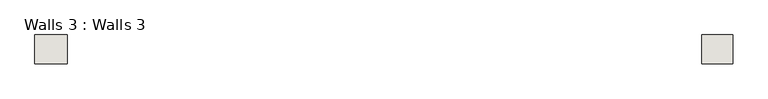
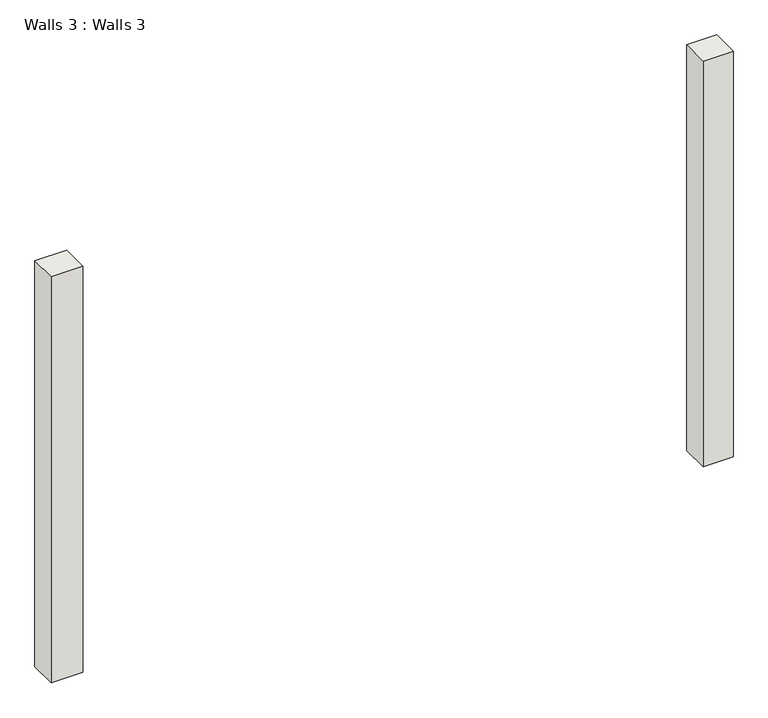
"""IFC4 building model written with IfcOpenShell, lengths in millimetres: wall geometry, Walls 3 : Walls 3."""

from ifc_helpers import new_model, si_unit, origin, origin_with_axes, place, context, project, spatial, polyline, outline, extrude, source, transform, mapped, element, save


def walls_3_walls_3_79010243(model_context):
    return source(origin(), model_context, "Body", "SweptSolid", [
        extrude(outline(polyline([(-7314.7803346, -3620.8536983), (-7540.7878119, -3620.8536983), (-7540.7878119, -3420.8536983), (-7314.7803346, -3420.8536983), (-7314.7803346, -3620.8536983)])), origin_with_axes(), (0.0, 0.0, 1.0), 3048.0),
        extrude(outline(polyline([(-2695.7378119, -3620.8536983), (-2909.3443924, -3620.8536983), (-2909.3443924, -3420.8536983), (-2695.7378119, -3420.8536983), (-2695.7378119, -3620.8536983)])), origin_with_axes(), (0.0, 0.0, 1.0), 3048.0),
    ])


if __name__ == "__main__":
    model = new_model("IFC4")
    model_context = context("Model", 3, world=origin())
    ifc_project = project(units=[si_unit("LENGTHUNIT", "METRE", prefix="MILLI")], contexts=[model_context])
    site = spatial("IfcSite", under=ifc_project)
    building = spatial("IfcBuilding", under=site)
    placement = place(None, origin())
    walls_3_walls_3_shape = walls_3_walls_3_79010243(model_context)
    element("IfcWall", 1, ObjectType="Walls 3 : Walls 3", at=placement, inside=building, context=model_context, shape_type="MappedRepresentation", body=[
        mapped(walls_3_walls_3_shape, transform((0.0, 0.0, 0.0), x_axis=(1.0, 0.0, 0.0), y_axis=(0.0, 1.0, 0.0), z_axis=(0.0, 0.0, 1.0))),
    ])
    save(model, "model.ifc")

# Revit data of these elements
# Element 1 (IfcWall, "Walls 3 : Walls 3")
#   Materials on its faces: "Default Wall"
# Materials
#   "Default Wall": colour RGB 80 80 80, transparency 0
